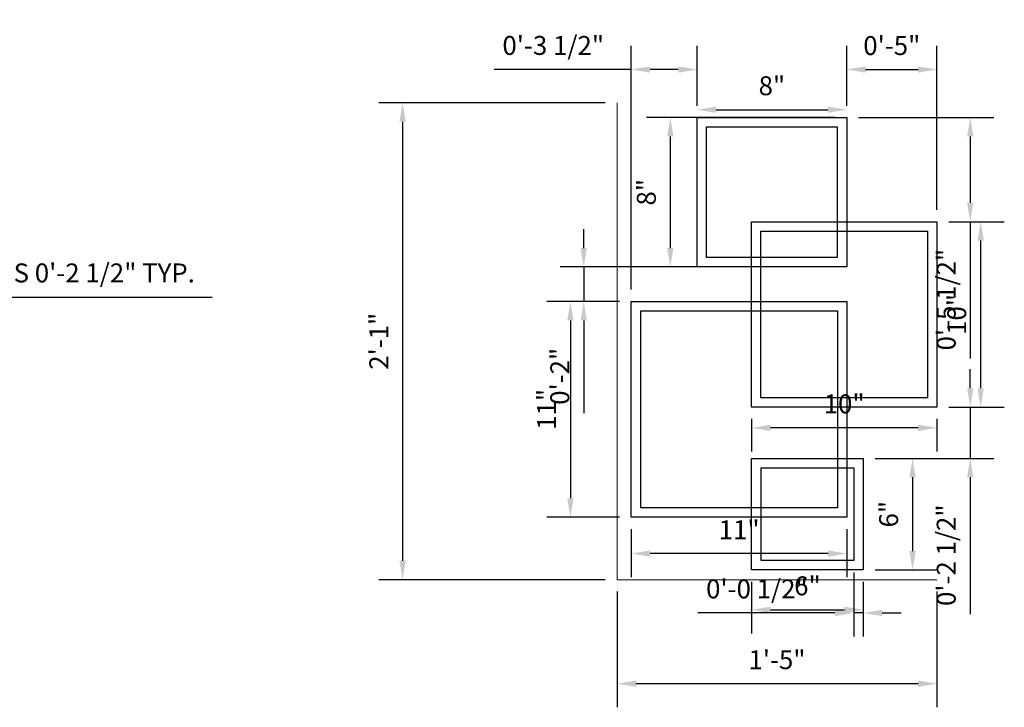
# Model space of a CAD drawing. Units: millimetres. Extents: x 7894 to 8038, y 6851 to 6951.
# Tile 49 of 49: x 7986 to 8038, y 6859 to 6896. Entities that reach past the tile are written whole.
import ezdxf

# ---------------------------------------------------------------- set-up
doc = ezdxf.new("R2010")
doc.units = ezdxf.units.MM
for name, color, linetype, lineweight in [('A-ANNO-DIMS', 2, 'Continuous', 18), ('A-DETL', 8, 'Continuous', 18), ('A-FURN-CASE', 7, 'Continuous', 30)]:
    doc.layers.add(name, color=color, linetype=linetype, lineweight=lineweight)
doc.styles.get("Standard").update_dxf_attribs({"font": 'arial.ttf'})
doc.dimstyles.new('ISO-25', dxfattribs={"dimtxt": 1, "dimasz": 1, "dimexe": 1.25, "dimexo": 0.625, "dimtad": 1, "dimdec": 0, "dimlunit": 4, "dimtxsty": 'Standard', "dimcen": 2.5, "dimclrt": 1, "dimadec": 0, "dimazin": 0, "dimtfac": 1, "dimtdec": 0, "dimtmove": 0, "dimatfit": 3, "dimfxl": 1, "dimarcsym": 0})

# ---------------------------------------------------------------- blocks, each defined once
blk = doc.blocks.new('*D1')
at = {"layer": 'A-ANNO-DIMS', "color": 0, "lineweight": -2, "transparency": 16777216}
for p, q in [((8021.8, 6891.099), (8021.8, 6892.138)), ((8029.7, 6891.099), (8029.7, 6892.138)), ((8022.8, 6890.888), (8028.7, 6890.888))]:
    blk.add_line(p, q, dxfattribs=at)
at = {"layer": 'A-ANNO-DIMS', "color": 0, "transparency": 16777216}
for points in [[(8022.8, 6891.054), (8022.8, 6890.721), (8021.8, 6890.888)], [(8028.7, 6891.054), (8028.7, 6890.721), (8029.7, 6890.888)]]:
    blk.add_solid(points, dxfattribs=at)
at = {"layer": 'Defpoints', "color": 0, "transparency": 16777216}
for p in [(8029.7, 6890.888), (8021.8, 6890.474), (8029.7, 6890.474)]:
    blk.add_point(p, dxfattribs=at)
at = {"layer": 'A-ANNO-DIMS', "color": 0, "transparency": 16777216, "insert": (8025.75, 6892.023), "char_height": 1, "attachment_point": 5}
blk.add_mtext('8"', dxfattribs=at)
blk = doc.blocks.new('*D2')
at = {"layer": 'A-ANNO-DIMS', "color": 0, "lineweight": -2, "transparency": 16777216}
for p, q in [((8029.075, 6890.474), (8019.131, 6890.474)), ((8020.381, 6889.474), (8020.381, 6883.574)), ((8029.075, 6882.574), (8019.131, 6882.574))]:
    blk.add_line(p, q, dxfattribs=at)
at = {"layer": 'A-ANNO-DIMS', "color": 0, "transparency": 16777216}
for points in [[(8020.214, 6889.474), (8020.548, 6889.474), (8020.381, 6890.474)], [(8020.214, 6883.574), (8020.548, 6883.574), (8020.381, 6882.574)]]:
    blk.add_solid(points, dxfattribs=at)
at = {"layer": 'Defpoints', "color": 0, "transparency": 16777216}
for p in [(8029.7, 6890.474), (8020.381, 6882.574), (8029.7, 6882.574)]:
    blk.add_point(p, dxfattribs=at)
at = {"layer": 'A-ANNO-DIMS', "color": 0, "transparency": 16777216, "insert": (8019.245, 6886.524), "char_height": 1, "attachment_point": 5, "rotation": 90}
blk.add_mtext('8"', dxfattribs=at)
blk = doc.blocks.new('*D3')
at = {"layer": 'A-ANNO-DIMS', "color": 0, "lineweight": -2, "transparency": 16777216}
for p, q in [((8035.094, 6884.968), (8038.029, 6884.968)), ((8036.779, 6883.968), (8036.779, 6876.168)), ((8035.094, 6875.168), (8038.029, 6875.168))]:
    blk.add_line(p, q, dxfattribs=at)
at = {"layer": 'A-ANNO-DIMS', "color": 0, "transparency": 16777216}
for points in [[(8036.612, 6883.968), (8036.945, 6883.968), (8036.779, 6884.968)], [(8036.612, 6876.168), (8036.945, 6876.168), (8036.779, 6875.168)]]:
    blk.add_solid(points, dxfattribs=at)
at = {"layer": 'Defpoints', "color": 0, "transparency": 16777216}
for p in [(8034.469, 6884.968), (8034.469, 6875.168), (8036.779, 6875.168)]:
    blk.add_point(p, dxfattribs=at)
at = {"layer": 'A-ANNO-DIMS', "color": 0, "transparency": 16777216, "insert": (8035.643, 6880.068), "char_height": 1, "attachment_point": 5, "rotation": 90}
blk.add_mtext('10"', dxfattribs=at)
blk = doc.blocks.new('*D4')
at = {"layer": 'A-ANNO-DIMS', "color": 0, "lineweight": -2, "transparency": 16777216}
for p, q in [((8024.669, 6874.543), (8024.669, 6872.823)), ((8034.469, 6874.543), (8034.469, 6872.823)), ((8033.469, 6874.073), (8025.669, 6874.073))]:
    blk.add_line(p, q, dxfattribs=at)
at = {"layer": 'A-ANNO-DIMS', "color": 0, "transparency": 16777216}
for points in [[(8025.669, 6874.24), (8025.669, 6873.907), (8024.669, 6874.073)], [(8033.469, 6874.24), (8033.469, 6873.907), (8034.469, 6874.073)]]:
    blk.add_solid(points, dxfattribs=at)
at = {"layer": 'Defpoints', "color": 0, "transparency": 16777216}
for p in [(8024.669, 6875.168), (8034.469, 6875.168), (8024.669, 6874.073)]:
    blk.add_point(p, dxfattribs=at)
at = {"layer": 'A-ANNO-DIMS', "color": 0, "transparency": 16777216, "insert": (8029.569, 6875.209), "char_height": 1, "attachment_point": 5}
blk.add_mtext('10"', dxfattribs=at)
blk = doc.blocks.new('*D5')
at = {"layer": 'A-ANNO-DIMS', "color": 0, "lineweight": -2, "transparency": 16777216}
for p, q in [((8031.202, 6872.462), (8034.431, 6872.462)), ((8033.181, 6871.462), (8033.181, 6867.562)), ((8031.202, 6866.562), (8034.431, 6866.562))]:
    blk.add_line(p, q, dxfattribs=at)
at = {"layer": 'A-ANNO-DIMS', "color": 0, "transparency": 16777216}
for points in [[(8033.015, 6871.462), (8033.348, 6871.462), (8033.181, 6872.462)], [(8033.015, 6867.562), (8033.348, 6867.562), (8033.181, 6866.562)]]:
    blk.add_solid(points, dxfattribs=at)
at = {"layer": 'Defpoints', "color": 0, "transparency": 16777216}
for p in [(8030.577, 6872.462), (8030.577, 6866.562), (8033.181, 6866.562)]:
    blk.add_point(p, dxfattribs=at)
at = {"layer": 'A-ANNO-DIMS', "color": 0, "transparency": 16777216, "insert": (8032.046, 6869.512), "char_height": 1, "attachment_point": 5, "rotation": 90}
blk.add_mtext('6"', dxfattribs=at)
blk = doc.blocks.new('*D6')
at = {"layer": 'A-ANNO-DIMS', "color": 0, "lineweight": -2, "transparency": 16777216}
for p, q in [((8024.677, 6865.937), (8024.677, 6863.206)), ((8030.577, 6865.937), (8030.577, 6863.206)), ((8025.677, 6864.456), (8029.577, 6864.456))]:
    blk.add_line(p, q, dxfattribs=at)
at = {"layer": 'A-ANNO-DIMS', "color": 0, "transparency": 16777216}
for points in [[(8025.677, 6864.623), (8025.677, 6864.29), (8024.677, 6864.456)], [(8029.577, 6864.623), (8029.577, 6864.29), (8030.577, 6864.456)]]:
    blk.add_solid(points, dxfattribs=at)
at = {"layer": 'Defpoints', "color": 0, "transparency": 16777216}
for p in [(8024.677, 6866.562), (8030.577, 6866.562), (8030.577, 6864.456)]:
    blk.add_point(p, dxfattribs=at)
at = {"layer": 'A-ANNO-DIMS', "color": 0, "transparency": 16777216, "insert": (8027.627, 6865.592), "char_height": 1, "attachment_point": 5}
blk.add_mtext('6"', dxfattribs=at)
blk = doc.blocks.new('*D7')
at = {"layer": 'A-ANNO-DIMS', "color": 0, "lineweight": -2, "transparency": 16777216}
for p, q in [((8017.692, 6880.751), (8013.853, 6880.751)), ((8015.103, 6879.751), (8015.103, 6870.351)), ((8017.692, 6869.351), (8013.853, 6869.351))]:
    blk.add_line(p, q, dxfattribs=at)
at = {"layer": 'A-ANNO-DIMS', "color": 0, "transparency": 16777216}
for points in [[(8014.937, 6879.751), (8015.27, 6879.751), (8015.103, 6880.751)], [(8014.937, 6870.351), (8015.27, 6870.351), (8015.103, 6869.351)]]:
    blk.add_solid(points, dxfattribs=at)
at = {"layer": 'Defpoints', "color": 0, "transparency": 16777216}
for p in [(8018.317, 6880.751), (8015.103, 6869.351), (8018.317, 6869.351)]:
    blk.add_point(p, dxfattribs=at)
at = {"layer": 'A-ANNO-DIMS', "color": 0, "transparency": 16777216, "insert": (8013.976, 6875.051), "char_height": 1, "attachment_point": 5, "rotation": 90}
blk.add_mtext('11"', dxfattribs=at)
blk = doc.blocks.new('*D8')
at = {"layer": 'A-ANNO-DIMS', "color": 0, "lineweight": -2, "transparency": 16777216}
for p, q in [((8018.317, 6868.726), (8018.317, 6866.18)), ((8029.717, 6868.726), (8029.717, 6866.18)), ((8028.717, 6867.43), (8019.317, 6867.43))]:
    blk.add_line(p, q, dxfattribs=at)
at = {"layer": 'A-ANNO-DIMS', "color": 0, "transparency": 16777216}
for points in [[(8019.317, 6867.597), (8019.317, 6867.264), (8018.317, 6867.43)], [(8028.717, 6867.597), (8028.717, 6867.264), (8029.717, 6867.43)]]:
    blk.add_solid(points, dxfattribs=at)
at = {"layer": 'Defpoints', "color": 0, "transparency": 16777216}
for p in [(8018.317, 6869.351), (8029.717, 6869.351), (8018.317, 6867.43)]:
    blk.add_point(p, dxfattribs=at)
at = {"layer": 'A-ANNO-DIMS', "color": 0, "transparency": 16777216, "insert": (8024.017, 6868.557), "char_height": 1, "attachment_point": 5}
blk.add_mtext('11"', dxfattribs=at)
blk = doc.blocks.new('*D9')
at = {"layer": 'A-ANNO-DIMS', "color": 0, "lineweight": -2, "transparency": 16777216}
for p, q in [((8017.569, 6865.425), (8017.569, 6859.304)), ((8034.469, 6865.425), (8034.469, 6859.304)), ((8018.569, 6860.554), (8033.469, 6860.554))]:
    blk.add_line(p, q, dxfattribs=at)
at = {"layer": 'A-ANNO-DIMS', "color": 0, "transparency": 16777216}
for points in [[(8018.569, 6860.721), (8018.569, 6860.388), (8017.569, 6860.554)], [(8033.469, 6860.721), (8033.469, 6860.388), (8034.469, 6860.554)]]:
    blk.add_solid(points, dxfattribs=at)
at = {"layer": 'Defpoints', "color": 0, "transparency": 16777216}
for p in [(8017.569, 6866.05), (8034.469, 6866.05), (8034.469, 6860.554)]:
    blk.add_point(p, dxfattribs=at)
at = {"layer": 'A-ANNO-DIMS', "color": 0, "transparency": 16777216, "insert": (8026.019, 6861.69), "char_height": 1, "attachment_point": 5}
blk.add_mtext('1\'-5"', dxfattribs=at)
blk = doc.blocks.new('*D10')
at = {"layer": 'A-ANNO-DIMS', "color": 0, "lineweight": -2, "transparency": 16777216}
for p, q in [((8016.944, 6891.25), (8004.988, 6891.25)), ((8006.238, 6890.25), (8006.238, 6867.05)), ((8016.944, 6866.05), (8004.988, 6866.05))]:
    blk.add_line(p, q, dxfattribs=at)
at = {"layer": 'A-ANNO-DIMS', "color": 0, "transparency": 16777216}
for points in [[(8006.072, 6890.25), (8006.405, 6890.25), (8006.238, 6891.25)], [(8006.072, 6867.05), (8006.405, 6867.05), (8006.238, 6866.05)]]:
    blk.add_solid(points, dxfattribs=at)
at = {"layer": 'Defpoints', "color": 0, "transparency": 16777216}
for p in [(8017.569, 6891.25), (8006.238, 6866.05), (8017.569, 6866.05)]:
    blk.add_point(p, dxfattribs=at)
at = {"layer": 'A-ANNO-DIMS', "color": 0, "transparency": 16777216, "insert": (8005.111, 6878.65), "char_height": 1, "attachment_point": 5, "rotation": 90}
blk.add_mtext('2\'-1"', dxfattribs=at)
blk = doc.blocks.new('BOX-SHELF-SMALL-ELEV')
for points in [[(0, 5.9), (5.9, 5.9), (5.9, 0), (0, 0)], [(0.5, 5.4), (5.4, 5.4), (5.4, 0.5), (0.5, 0.5)]]:
    blk.add_lwpolyline(points, close=True)
blk = doc.blocks.new('*D19')
at = {"layer": 'A-ANNO-DIMS', "color": 0, "lineweight": -2, "transparency": 16777216}
for p, q in [((7975.917, 6880.988), (7974.917, 6880.988)), ((7976.917, 6880.988), (7979.357, 6880.988)), ((7980.357, 6880.988), (7996.183, 6880.988)), ((7976.917, 6880.729), (7976.917, 6879.738)), ((7979.357, 6880.729), (7979.357, 6879.738))]:
    blk.add_line(p, q, dxfattribs=at)
at = {"layer": 'A-ANNO-DIMS', "color": 0, "transparency": 16777216}
for points in [[(7975.917, 6881.155), (7975.917, 6880.822), (7976.917, 6880.988)], [(7980.357, 6881.155), (7980.357, 6880.822), (7979.357, 6880.988)]]:
    blk.add_solid(points, dxfattribs=at)
at = {"layer": 'Defpoints', "color": 0, "transparency": 16777216}
for p in [(7976.917, 6881.354), (7979.357, 6881.354), (7979.357, 6880.988)]:
    blk.add_point(p, dxfattribs=at)
at = {"layer": 'A-ANNO-DIMS', "color": 1, "transparency": 16777216, "insert": (7988.77, 6882.131), "char_height": 1, "attachment_point": 5}
blk.add_mtext('REEDS 0\'-2 1/2" TYP.', dxfattribs=at)
blk = doc.blocks.new('*D47')
at = {"layer": 'A-ANNO-DIMS', "color": 0, "lineweight": -2, "transparency": 16777216}
for p, q in [((8015.809, 6883.574), (8015.809, 6884.574)), ((8021.175, 6882.574), (8014.559, 6882.574)), ((8015.809, 6882.574), (8015.809, 6880.751)), ((8017.692, 6880.751), (8014.559, 6880.751)), ((8015.809, 6879.751), (8015.809, 6874.843))]:
    blk.add_line(p, q, dxfattribs=at)
at = {"layer": 'A-ANNO-DIMS', "color": 0, "transparency": 16777216}
for points in [[(8015.642, 6883.574), (8015.975, 6883.574), (8015.809, 6882.574)], [(8015.642, 6879.751), (8015.975, 6879.751), (8015.809, 6880.751)]]:
    blk.add_solid(points, dxfattribs=at)
at = {"layer": 'Defpoints', "color": 0, "transparency": 16777216}
for p in [(8021.8, 6882.574), (8015.809, 6880.751), (8018.317, 6880.751)]:
    blk.add_point(p, dxfattribs=at)
at = {"layer": 'A-ANNO-DIMS', "color": 1, "transparency": 16777216, "insert": (8014.673, 6876.797), "char_height": 1, "attachment_point": 5, "rotation": 90}
blk.add_mtext('0\'-2"', dxfattribs=at)
blk = doc.blocks.new('*D48')
at = {"layer": 'A-ANNO-DIMS', "color": 0, "lineweight": -2, "transparency": 16777216}
for p, q in [((8036.229, 6876.168), (8036.229, 6877.168)), ((8035.094, 6875.168), (8037.479, 6875.168)), ((8036.229, 6875.168), (8036.229, 6872.462)), ((8031.202, 6872.462), (8037.479, 6872.462)), ((8036.229, 6871.462), (8036.229, 6864.223))]:
    blk.add_line(p, q, dxfattribs=at)
at = {"layer": 'A-ANNO-DIMS', "color": 0, "transparency": 16777216}
for points in [[(8036.062, 6876.168), (8036.395, 6876.168), (8036.229, 6875.168)], [(8036.062, 6871.462), (8036.395, 6871.462), (8036.229, 6872.462)]]:
    blk.add_solid(points, dxfattribs=at)
at = {"layer": 'Defpoints', "color": 0, "transparency": 16777216}
for p in [(8034.469, 6875.168), (8030.577, 6872.462), (8036.229, 6872.462)]:
    blk.add_point(p, dxfattribs=at)
at = {"layer": 'A-ANNO-DIMS', "color": 1, "transparency": 16777216, "insert": (8035.087, 6867.343), "char_height": 1, "attachment_point": 5, "rotation": 90}
blk.add_mtext('0\'-2 1/2"', dxfattribs=at)
blk = doc.blocks.new('*D49')
at = {"layer": 'A-ANNO-DIMS', "color": 0, "lineweight": -2, "transparency": 16777216}
for p, q in [((8018.317, 6881.376), (8018.317, 6894.26)), ((8021.8, 6891.099), (8021.8, 6894.26)), ((8018.317, 6893.01), (8011.079, 6893.01)), ((8020.8, 6893.01), (8019.317, 6893.01))]:
    blk.add_line(p, q, dxfattribs=at)
at = {"layer": 'A-ANNO-DIMS', "color": 0, "transparency": 16777216}
for points in [[(8019.317, 6893.176), (8019.317, 6892.843), (8018.317, 6893.01)], [(8020.8, 6893.176), (8020.8, 6892.843), (8021.8, 6893.01)]]:
    blk.add_solid(points, dxfattribs=at)
at = {"layer": 'Defpoints', "color": 0, "transparency": 16777216}
for p in [(8018.317, 6893.01), (8021.8, 6890.474), (8018.317, 6880.751)]:
    blk.add_point(p, dxfattribs=at)
at = {"layer": 'A-ANNO-DIMS', "color": 1, "transparency": 16777216, "insert": (8014.198, 6894.152), "char_height": 1, "attachment_point": 5}
blk.add_mtext('0\'-3 1/2"', dxfattribs=at)
blk = doc.blocks.new('*D50')
at = {"layer": 'A-ANNO-DIMS', "color": 0, "lineweight": -2, "transparency": 16777216}
for p, q in [((8029.7, 6891.099), (8029.7, 6894.26)), ((8034.469, 6885.593), (8034.469, 6894.26)), ((8030.7, 6893.01), (8033.469, 6893.01))]:
    blk.add_line(p, q, dxfattribs=at)
at = {"layer": 'A-ANNO-DIMS', "color": 0, "transparency": 16777216}
for points in [[(8030.7, 6893.176), (8030.7, 6892.843), (8029.7, 6893.01)], [(8033.469, 6893.176), (8033.469, 6892.843), (8034.469, 6893.01)]]:
    blk.add_solid(points, dxfattribs=at)
at = {"layer": 'Defpoints', "color": 0, "transparency": 16777216}
for p in [(8034.469, 6893.01), (8029.7, 6890.474), (8034.469, 6884.968)]:
    blk.add_point(p, dxfattribs=at)
at = {"layer": 'A-ANNO-DIMS', "color": 1, "transparency": 16777216, "insert": (8032.085, 6894.145), "char_height": 1, "attachment_point": 5}
blk.add_mtext('0\'-5"', dxfattribs=at)
blk = doc.blocks.new('*D51')
at = {"layer": 'A-ANNO-DIMS', "color": 0, "lineweight": -2, "transparency": 16777216}
for p, q in [((8030.325, 6890.474), (8037.479, 6890.474)), ((8036.229, 6889.474), (8036.229, 6885.968)), ((8035.094, 6884.968), (8037.479, 6884.968)), ((8036.229, 6884.968), (8036.229, 6877.73))]:
    blk.add_line(p, q, dxfattribs=at)
at = {"layer": 'A-ANNO-DIMS', "color": 0, "transparency": 16777216}
for points in [[(8036.062, 6889.474), (8036.395, 6889.474), (8036.229, 6890.474)], [(8036.062, 6885.968), (8036.395, 6885.968), (8036.229, 6884.968)]]:
    blk.add_solid(points, dxfattribs=at)
at = {"layer": 'Defpoints', "color": 0, "transparency": 16777216}
for p in [(8029.7, 6890.474), (8034.469, 6884.968), (8036.229, 6884.968)]:
    blk.add_point(p, dxfattribs=at)
at = {"layer": 'A-ANNO-DIMS', "color": 1, "transparency": 16777216, "insert": (8035.087, 6880.849), "char_height": 1, "attachment_point": 5, "rotation": 90}
blk.add_mtext('0\'-5 1/2"', dxfattribs=at)
blk = doc.blocks.new('*D52')
at = {"layer": 'A-ANNO-DIMS', "color": 0, "lineweight": -2, "transparency": 16777216}
for p, q in [((8030.077, 6866.437), (8030.077, 6863.04)), ((8030.577, 6865.937), (8030.577, 6863.04)), ((8029.077, 6864.29), (8021.838, 6864.29)), ((8030.577, 6864.29), (8030.077, 6864.29)), ((8031.577, 6864.29), (8032.577, 6864.29))]:
    blk.add_line(p, q, dxfattribs=at)
at = {"layer": 'A-ANNO-DIMS', "color": 0, "transparency": 16777216}
for points in [[(8029.077, 6864.456), (8029.077, 6864.123), (8030.077, 6864.29)], [(8031.577, 6864.456), (8031.577, 6864.123), (8030.577, 6864.29)]]:
    blk.add_solid(points, dxfattribs=at)
at = {"layer": 'Defpoints', "color": 0, "transparency": 16777216}
for p in [(8030.077, 6867.062), (8030.577, 6866.562), (8030.077, 6864.29)]:
    blk.add_point(p, dxfattribs=at)
at = {"layer": 'A-ANNO-DIMS', "color": 1, "transparency": 16777216, "insert": (8024.958, 6865.432), "char_height": 1, "attachment_point": 5}
blk.add_mtext('0\'-0 1/2"', dxfattribs=at)

msp = doc.modelspace()

# ---------------------------------------------------------------- linework, layer by layer
at = {"layer": 'A-DETL'}
for p in [(8017.569, 6891.25), (8034.469, 6866.05)]:
    msp.add_line(p, (8017.569, 6866.05), dxfattribs=at)
at = {"layer": 'A-FURN-CASE'}
for points in [[(8021.8, 6890.474), (8029.7, 6890.474), (8029.7, 6882.574), (8021.8, 6882.574)], [(8022.3, 6889.974), (8029.2, 6889.974), (8029.2, 6883.074), (8022.3, 6883.074)], [(8024.669, 6884.968), (8034.469, 6884.968), (8034.469, 6875.168), (8024.669, 6875.168)], [(8025.169, 6884.468), (8033.969, 6884.468), (8033.969, 6875.668), (8025.169, 6875.668)], [(8018.317, 6880.751), (8029.717, 6880.751), (8029.717, 6869.351), (8018.317, 6869.351)], [(8018.817, 6880.251), (8029.217, 6880.251), (8029.217, 6869.851), (8018.817, 6869.851)]]:
    msp.add_lwpolyline(points, close=True, dxfattribs=at)

# ---------------------------------------------------------------- block references
msp.add_blockref('BOX-SHELF-SMALL-ELEV', (8024.677, 6866.562), dxfattribs=at)

# ---------------------------------------------------------------- dimensions: what is measured, and where the dimension line sits
at = {"layer": 'A-ANNO-DIMS'}
for base, p1, p2, override, picture, middle in [((8018.317, 6893.01), (8021.8, 6890.474), (8018.317, 6880.751), {"dimdec": 1, "dimlfac": 1, "dimrnd": 0, "dimzin": 1, "dimdsep": 46, "dimlunit": 4, "dimfrac": 2}, '*D49', (8014.198, 6894.152)), ((8034.469, 6893.01), (8029.7, 6890.474), (8034.469, 6884.968), {"dimdec": 1, "dimlfac": 1, "dimrnd": 0, "dimzin": 1, "dimdsep": 46, "dimlunit": 4, "dimfrac": 2}, '*D50', (8032.085, 6894.145)), ((8029.7, 6890.888), (8021.8, 6890.474), (8029.7, 6890.474), {"dimclrd": 0, "dimclre": 0, "dimclrt": 0}, '*D1', (8025.75, 6892.023)), ((8024.669, 6874.073), (8034.469, 6875.168), (8024.669, 6875.168), {"dimclrd": 0, "dimclre": 0, "dimclrt": 0}, '*D4', (8029.569, 6875.209)), ((8018.317, 6867.43), (8029.717, 6869.351), (8018.317, 6869.351), {"dimclrd": 0, "dimclre": 0, "dimclrt": 0}, '*D8', (8024.017, 6868.557)), ((8030.077, 6864.29), (8030.577, 6866.562), (8030.077, 6867.062), {"dimdec": 1, "dimlfac": 1, "dimrnd": 0, "dimzin": 1, "dimdsep": 46, "dimlunit": 4, "dimfrac": 2}, '*D52', (8024.958, 6865.432)), ((8030.577, 6864.456), (8024.677, 6866.562), (8030.577, 6866.562), {"dimclrd": 0, "dimclre": 0, "dimclrt": 0}, '*D6', (8027.627, 6865.592)), ((8034.469, 6860.554), (8017.569, 6866.05), (8034.469, 6866.05), {"dimclrd": 0, "dimclre": 0, "dimclrt": 0}, '*D9', (8026.019, 6861.69))]:
    dim = msp.add_linear_dim(base=base, p1=p1, p2=p2, dimstyle='ISO-25', override=override, dxfattribs=at)
    dim.commit()
    dim.dimension.update_dxf_attribs({"geometry": picture, "text_midpoint": middle})
for base, p1, p2, override, picture, middle in [((8006.238, 6866.05), (8017.569, 6891.25), (8017.569, 6866.05), {"dimclrd": 0, "dimclre": 0, "dimclrt": 0}, '*D10', (8005.111, 6878.65)), ((8020.381, 6882.574), (8029.7, 6890.474), (8029.7, 6882.574), {"dimclrd": 0, "dimclre": 0, "dimclrt": 0}, '*D2', (8019.245, 6886.524)), ((8036.229, 6884.968), (8029.7, 6890.474), (8034.469, 6884.968), {"dimdec": 1, "dimlfac": 1, "dimrnd": 0, "dimzin": 1, "dimdsep": 46, "dimlunit": 4, "dimfrac": 2}, '*D51', (8035.087, 6880.849)), ((8036.779, 6875.168), (8034.469, 6884.968), (8034.469, 6875.168), {"dimclrd": 0, "dimclre": 0, "dimclrt": 0}, '*D3', (8035.643, 6880.068)), ((8015.809, 6880.751), (8021.8, 6882.574), (8018.317, 6880.751), {"dimdec": 1, "dimlfac": 1, "dimrnd": 0, "dimzin": 1, "dimdsep": 46, "dimlunit": 4, "dimfrac": 2}, '*D47', (8014.673, 6876.797)), ((8015.103, 6869.351), (8018.317, 6880.751), (8018.317, 6869.351), {"dimclrd": 0, "dimclre": 0, "dimclrt": 0}, '*D7', (8013.976, 6875.051)), ((8036.229, 6872.462), (8034.469, 6875.168), (8030.577, 6872.462), {"dimdec": 1, "dimlfac": 1, "dimrnd": 0, "dimzin": 1, "dimdsep": 46, "dimlunit": 4, "dimfrac": 2}, '*D48', (8035.087, 6867.343)), ((8033.181, 6866.562), (8030.577, 6872.462), (8030.577, 6866.562), {"dimclrd": 0, "dimclre": 0, "dimclrt": 0}, '*D5', (8032.046, 6869.512))]:
    dim = msp.add_linear_dim(base=base, p1=p1, p2=p2, angle=90, dimstyle='ISO-25', override=override, dxfattribs=at)
    dim.commit()
    dim.dimension.update_dxf_attribs({"geometry": picture, "text_midpoint": middle})
dim = msp.add_linear_dim(base=(7979.357, 6880.988), p1=(7976.917, 6881.354), p2=(7979.357, 6881.354), text='REEDS <> TYP.', dimstyle='ISO-25', override={"dimdec": 1, "dimlfac": 1, "dimrnd": 0, "dimzin": 1, "dimdsep": 46, "dimlunit": 4, "dimfrac": 2}, dxfattribs=at)
dim.commit()
dim.dimension.update_dxf_attribs({"geometry": '*D19', "text_midpoint": (7988.77, 6882.131)})

doc.saveas('drawing.dxf')
